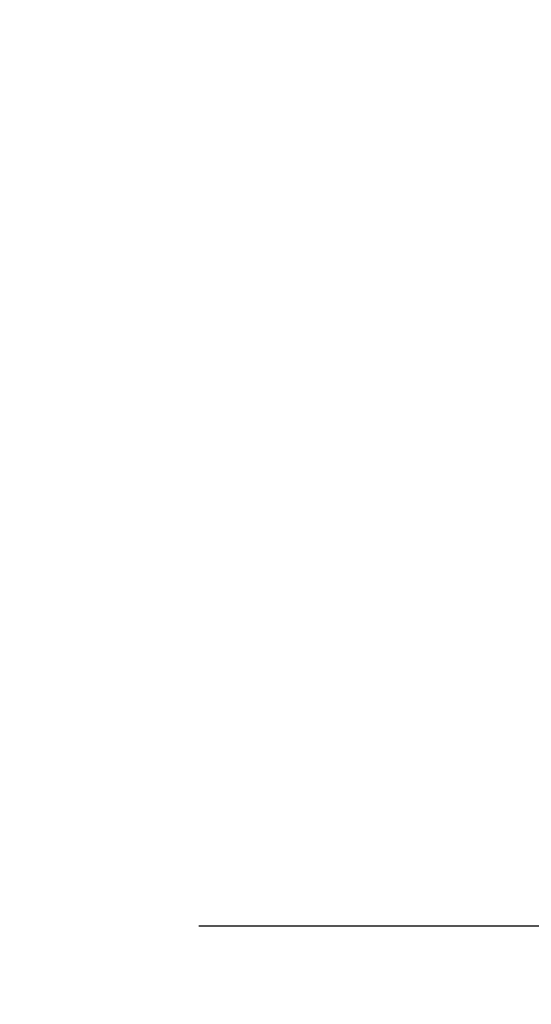
# Model space of a CAD drawing. Units: inches. Extents: x 2083 to 3317, y 1141 to 2115.
# Tile 215 of 256: x 3127.208 to 3128.284, y 1263.096 to 1265.165. Entities that reach past the tile are written whole.
import ezdxf

# ---------------------------------------------------------------- set-up
doc = ezdxf.new("R2010")
doc.units = ezdxf.units.IN
doc.layers.add('A-ANNO-DIMS', color=2, linetype='Continuous', lineweight=18)
doc.styles.get("Standard").update_dxf_attribs({"font": 'arial.ttf'})
doc.dimstyles.new('ISO-25', dxfattribs={"dimtxt": 12, "dimasz": 12, "dimexe": 1.25, "dimexo": 0.625, "dimtad": 1, "dimlunit": 3, "dimtxsty": 'Standard', "dimcen": 2.5, "dimadec": 0, "dimazin": 0, "dimtfac": 1, "dimtmove": 0, "dimatfit": 3, "dimfxl": 1, "dimarcsym": 0})

# ---------------------------------------------------------------- blocks, each defined once
blk = doc.blocks.new('*D9')
at = {"layer": 'A-ANNO-DIMS', "color": 0, "lineweight": -2, "transparency": 16777216}
for p, q in [((3127.5848, 1486.7614), (3190.4031, 1486.7614)), ((3189.1531, 1474.7614), (3189.1531, 1275.2614)), ((3127.5848, 1263.2614), (3190.4031, 1263.2614))]:
    blk.add_line(p, q, dxfattribs=at)
at = {"layer": 'A-ANNO-DIMS', "color": 0, "transparency": 16777216}
for points in [[(3187.1531, 1474.7614), (3191.1531, 1474.7614), (3189.1531, 1486.7614)], [(3187.1531, 1275.2614), (3191.1531, 1275.2614), (3189.1531, 1263.2614)]]:
    blk.add_solid(points, dxfattribs=at)
at = {"layer": 'Defpoints', "color": 0, "transparency": 16777216}
for p in [(3126.9598, 1486.7614), (3126.9598, 1263.2614), (3189.1531, 1263.2614)]:
    blk.add_point(p, dxfattribs=at)
at = {"layer": 'A-ANNO-DIMS', "color": 0, "transparency": 16777216, "insert": (3182.4012, 1375.0114), "char_height": 12, "attachment_point": 5, "rotation": 90}
blk.add_mtext('18\'-7.5"', dxfattribs=at)
blk = doc.blocks.new('*D26')
at = {"layer": 'A-ANNO-DIMS', "color": 0, "lineweight": -2, "transparency": 16777216}
for p, q in [((3088.9858, 1274.9151), (3088.9858, 1270.952)), ((3111.24, 1274.9151), (3111.24, 1270.952)), ((3076.9858, 1272.202), (2840.2624, 1272.202)), ((3111.24, 1272.202), (3088.9858, 1272.202)), ((3123.24, 1272.202), (3135.24, 1272.202))]:
    blk.add_line(p, q, dxfattribs=at)
at = {"layer": 'A-ANNO-DIMS', "color": 0, "transparency": 16777216}
for points in [[(3076.9858, 1274.202), (3076.9858, 1270.202), (3088.9858, 1272.202)], [(3123.24, 1274.202), (3123.24, 1270.202), (3111.24, 1272.202)]]:
    blk.add_solid(points, dxfattribs=at)
at = {"layer": 'Defpoints', "color": 0, "transparency": 16777216}
for p in [(3088.9858, 1275.5401), (3111.24, 1275.5401), (3088.9858, 1272.202)]:
    blk.add_point(p, dxfattribs=at)
at = {"layer": 'A-ANNO-DIMS', "color": 0, "transparency": 16777216, "insert": (2952.6241, 1279.0316), "char_height": 12, "attachment_point": 5}
blk.add_mtext('NIGHTSTAND 1\'-10 1/2" TYP.', dxfattribs=at)
blk = doc.blocks.new('*D27')
at = {"layer": 'A-ANNO-DIMS', "color": 0, "lineweight": -2, "transparency": 16777216}
for p, q in [((3114.5782, 1309.7943), (3114.5782, 1321.7943)), ((3111.865, 1297.7943), (3115.8282, 1297.7943)), ((3114.5782, 1297.7943), (3114.5782, 1275.5401)), ((3111.865, 1275.5401), (3115.8282, 1275.5401)), ((3114.5782, 1263.5401), (3114.5782, 1140.9886))]:
    blk.add_line(p, q, dxfattribs=at)
at = {"layer": 'A-ANNO-DIMS', "color": 0, "transparency": 16777216}
for points in [[(3112.5782, 1309.7943), (3116.5782, 1309.7943), (3114.5782, 1297.7943)], [(3112.5782, 1263.5401), (3116.5782, 1263.5401), (3114.5782, 1275.5401)]]:
    blk.add_solid(points, dxfattribs=at)
at = {"layer": 'Defpoints', "color": 0, "transparency": 16777216}
for p in [(3111.24, 1297.7943), (3111.24, 1275.5401), (3114.5782, 1275.5401)]:
    blk.add_point(p, dxfattribs=at)
at = {"layer": 'A-ANNO-DIMS', "color": 0, "transparency": 16777216, "insert": (3107.7485, 1196.2643), "char_height": 12, "attachment_point": 5, "rotation": 90}
blk.add_mtext('1\'-10 1/2" TYP.', dxfattribs=at)
blk = doc.blocks.new('*D35')
at = {"layer": 'A-ANNO-DIMS', "color": 0, "lineweight": -2, "transparency": 16777216}
for p, q in [((3127.5848, 2020.7614), (3180.5598, 2020.7614)), ((3179.3098, 1275.2614), (3179.3098, 2008.7614)), ((3127.5848, 1263.2614), (3180.5598, 1263.2614))]:
    blk.add_line(p, q, dxfattribs=at)
at = {"layer": 'A-ANNO-DIMS', "color": 0, "transparency": 16777216}
for points in [[(3177.3098, 2008.7614), (3181.3098, 2008.7614), (3179.3098, 2020.7614)], [(3177.3098, 1275.2614), (3181.3098, 1275.2614), (3179.3098, 1263.2614)]]:
    blk.add_solid(points, dxfattribs=at)
at = {"layer": 'Defpoints', "color": 0, "transparency": 16777216}
for p in [(3126.9598, 2020.7614), (3179.3098, 2020.7614), (3126.9598, 1263.2614)]:
    blk.add_point(p, dxfattribs=at)
at = {"layer": 'A-ANNO-DIMS', "color": 0, "transparency": 16777216, "insert": (3172.4761, 1642.0114), "char_height": 12, "attachment_point": 5, "rotation": 90}
blk.add_mtext('63\'-1 1/2"', dxfattribs=at)

msp = doc.modelspace()

# ---------------------------------------------------------------- dimensions: what is measured, and where the dimension line sits
at = {"layer": 'A-ANNO-DIMS'}
for base, p1, p2, override, picture, middle in [((3179.3098, 2020.7614), (3126.9598, 1263.2614), (3126.9598, 2020.7614), {"dimdec": 1, "dimlfac": 1, "dimrnd": 0, "dimzin": 1, "dimdsep": 46, "dimlunit": 4, "dimfrac": 2}, '*D35', (3172.4761, 1642.0114)), ((3189.1531, 1263.2614), (3126.9598, 1486.7614), (3126.9598, 1263.2614), {"dimclrd": 0, "dimclre": 0, "dimclrt": 0}, '*D9', (3182.4012, 1375.0114))]:
    dim = msp.add_linear_dim(base=base, p1=p1, p2=p2, angle=90, dimstyle='ISO-25', override=override, dxfattribs=at)
    dim.commit()
    dim.dimension.update_dxf_attribs({"geometry": picture, "text_midpoint": middle})
for base, p1, p2, angle, text, picture, middle in [((3114.5782, 1275.5401), (3111.24, 1297.7943), (3111.24, 1275.5401), 270, '<> TYP.', '*D27', (3107.7485, 1196.2643)), ((3088.9858, 1272.202), (3111.24, 1275.5401), (3088.9858, 1275.5401), 180, 'NIGHTSTAND <> TYP.', '*D26', (2952.6241, 1279.0316))]:
    dim = msp.add_linear_dim(base=base, p1=p1, p2=p2, angle=angle, text=text, dimstyle='ISO-25', override={"dimdec": 1, "dimlfac": 1, "dimrnd": 0, "dimzin": 1, "dimdsep": 46, "dimlunit": 4, "dimfrac": 2}, dxfattribs=at)
    dim.commit()
    dim.dimension.update_dxf_attribs({"geometry": picture, "text_midpoint": middle})

doc.saveas('drawing.dxf')
